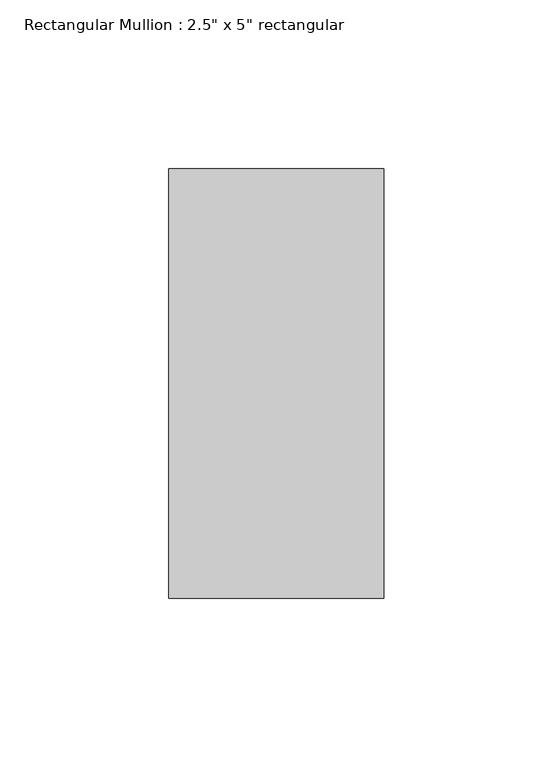
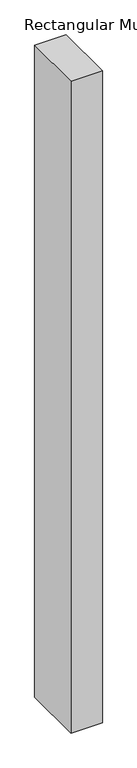
"""IFC4 building model written with IfcOpenShell, lengths in millimetres: member geometry."""

from ifc_helpers import new_model, si_unit, frame, origin, place, context, project, spatial, polyline, outline, extrude, source, transform, mapped, element, save


def member_16a3b7c2(model_context):
    return source(origin(), model_context, "Body", "SweptSolid", [
        extrude(outline(polyline([(0.0, 63.5), (0.0, -63.5), (-63.5, -63.5), (-63.5, 63.5), (0.0, 63.5)])), frame((0.0, 0.0, -1394.8833333), z_axis=(0.0, 0.0, 1.0), x_axis=(1.0, 0.0, 0.0)), (0.0, 0.0, 1.0), 1394.8833333),
    ])


if __name__ == "__main__":
    model = new_model("IFC4")
    model_context = context("Model", 3, world=origin())
    ifc_project = project(units=[si_unit("LENGTHUNIT", "METRE", prefix="MILLI")], contexts=[model_context])
    site = spatial("IfcSite", under=ifc_project)
    building = spatial("IfcBuilding", under=site)
    placement = place(None, origin())
    member_shape = member_16a3b7c2(model_context)
    element("IfcMember", 1, ObjectType="Rectangular Mullion : 2.5\" x 5\" rectangular", at=placement, inside=building, context=model_context, shape_type="MappedRepresentation", body=[
        mapped(member_shape, transform((0.0, 0.0, 0.0), x_axis=(1.0, 0.0, 0.0), y_axis=(0.0, 1.0, 0.0), z_axis=(0.0, 0.0, 1.0))),
    ])
    save(model, "model.ifc")

# Revit data of these elements
# Type "Rectangular Mullion : 2.5\" x 5\" rectangular"
#   built-in parameter 1007304 = 0.416667 (stored number, unit not read)
#   built-in parameter 1007301 = 0.104167 (stored number, unit not read)
#   built-in parameter 1007300 = 0.104167 (stored number, unit not read)
# Element 1 (IfcMember, "Rectangular Mullion : 2.5\" x 5\" rectangular")
#   Materials on its faces: "Aluminum"
# Materials
#   "Aluminum": class "Metal", colour RGB 247 247 247, transparency 0, Description = "Aluminum 6061", Cost = 0
